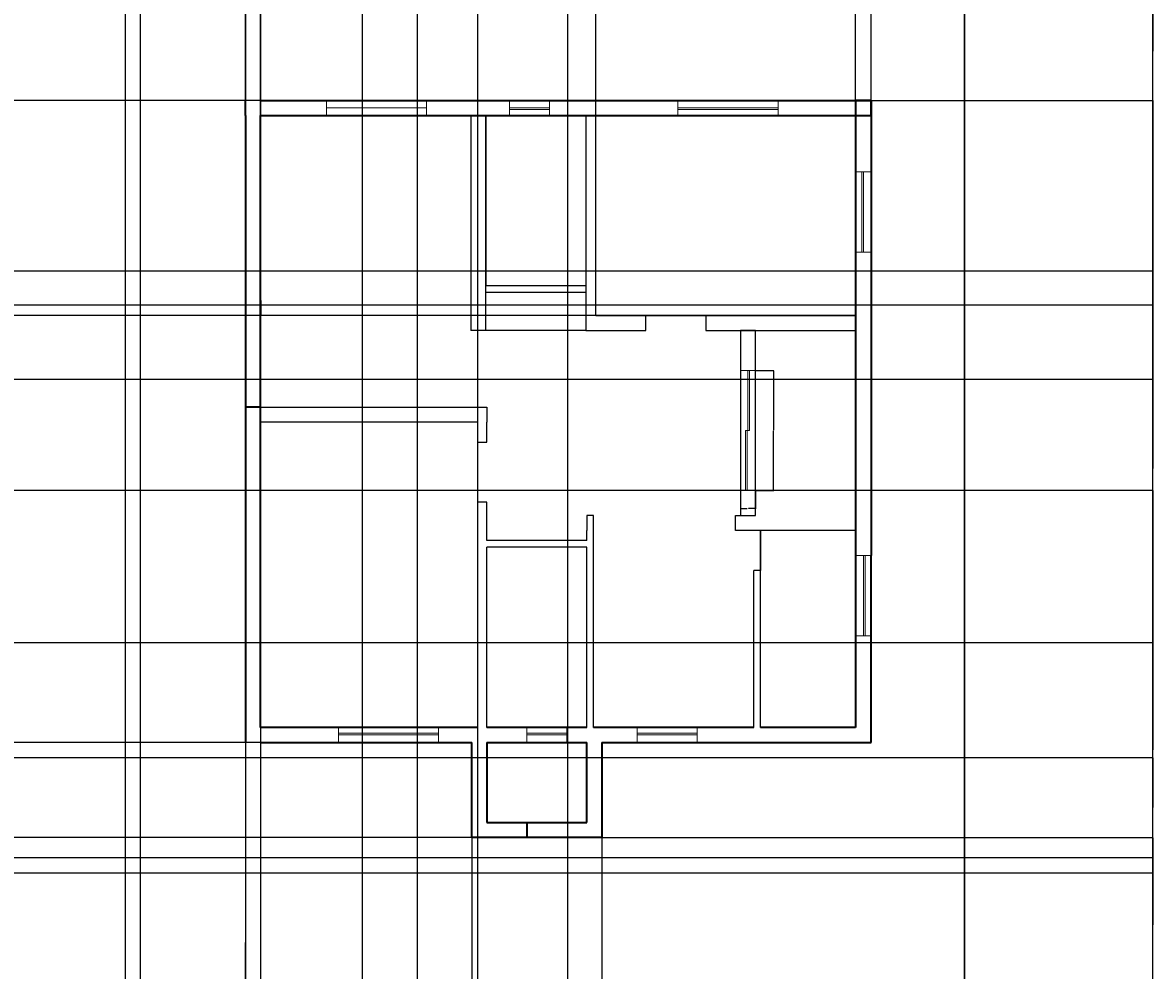
# Model space of a CAD drawing. Units: inches. Extents: x 2029 to 8798, y 1998 to 6373.
# Tile 7 of 11: x 3826 to 4504, y 4599 to 5168. Entities that reach past the tile are written whole.
import ezdxf

# ---------------------------------------------------------------- set-up
doc = ezdxf.new("R2010")
doc.units = ezdxf.units.IN
for name, color, linetype, lineweight in [('A-ANNO-DIMS', 2, 'Continuous', 18), ('A-GLAZ', 4, 'Continuous', 18), ('A-WALL-CIRC', 7, 'Continuous', 25), ('A-WALL-EXTR', 7, 'Continuous', 35), ('A-WALL-INTR', 7, 'Continuous', 25)]:
    doc.layers.add(name, color=color, linetype=linetype, lineweight=lineweight)
doc.styles.get("Standard").update_dxf_attribs({"font": 'arial.ttf'})
doc.dimstyles.get("Standard").update_dxf_attribs({"dimtxt": 0.18, "dimasz": 0.18, "dimexe": 0.18, "dimexo": 0.0625, "dimgap": 0.09, "dimtad": 0, "dimtih": 1, "dimtoh": 1, "dimdec": 4, "dimzin": 0, "dimdsep": 46, "dimtxsty": 'Standard', "dimcen": 0.09, "dimadec": 0, "dimazin": 0, "dimtfac": 1, "dimtdec": 4, "dimtofl": 0, "dimtmove": 0, "dimatfit": 3, "dimfxl": 1, "dimtolj": 1, "dimtzin": 0, "dimarcsym": 0})

# ---------------------------------------------------------------- blocks, each defined once
blk = doc.blocks.new('WIN-60')
for p, q in [((0, 0), (0, 9)), ((60, 9), (60, 0)), ((0, 4.5), (60, 4.5)), ((0, 3.5), (60, 3.5))]:
    blk.add_line(p, q)
blk = doc.blocks.new('WIN-36')
for p, q in [((0, 36), (9, 36)), ((3.5, 36), (3.5, 0)), ((4.5, 36), (4.5, 0)), ((9, 0), (0, 0))]:
    blk.add_line(p, q)
blk = doc.blocks.new('WIN-24')
for p, q in [((0, 0), (0, 9)), ((24, 9), (24, 0)), ((0, 4.5), (24, 4.5)), ((0, 3.5), (24, 3.5))]:
    blk.add_line(p, q)
blk = doc.blocks.new('WIN-48-DEEP-JAMB')
for p, q in [((9.38, 48), (0, 48)), ((0, 48), (0, 0)), ((3.69, 48), (3.69, 0)), ((4.69, 48), (4.69, 0)), ((0, 0), (9.38, 0))]:
    blk.add_line(p, q)
blk = doc.blocks.new('GLAZ-SLIDER-72-V')
for p, q in [((0, 72), (9, 72)), ((4.5, 72), (4.5, 36)), ((5.5, 72), (5.5, 36)), ((9, 72), (9, 0)), ((3, 36), (3, 0)), ((3, 36), (4, 36)), ((4, 36), (4, 0)), ((4.5, 36), (5.5, 36)), ((9, 0), (0, 0))]:
    blk.add_line(p, q)
blk = doc.blocks.new('WIN-60-SINGLE-LINE')
for p, q in [((0, 0), (0, 9)), ((0, 9), (60, 9)), ((60, 9), (60, 0)), ((0, 4.5), (60, 4.5))]:
    blk.add_line(p, q)
blk = doc.blocks.new('*D25')
at = {"layer": 'A-ANNO-DIMS', "color": 0, "lineweight": -2, "transparency": 16777216}
for p, q in [((4265.45, 4959.09), (4276.37, 4959.09)), ((4276.19, 4958.91), (4276.19, 4923.28)), ((4276.19, 4887.27), (4276.19, 4922.91)), ((4265.45, 4887.09), (4276.37, 4887.09))]:
    blk.add_line(p, q, dxfattribs=at)
at = {"layer": 'A-ANNO-DIMS', "color": 0, "transparency": 16777216}
for points in [[(4276.16, 4958.91), (4276.22, 4958.91), (4276.19, 4959.09)], [(4276.16, 4887.27), (4276.22, 4887.27), (4276.19, 4887.09)]]:
    blk.add_solid(points, dxfattribs=at)
at = {"layer": 'Defpoints', "color": 0, "transparency": 16777216}
for p in [(4265.39, 4959.09), (4276.19, 4959.09), (4265.39, 4887.09)]:
    blk.add_point(p, dxfattribs=at)
at = {"layer": 'A-ANNO-DIMS', "color": 0, "transparency": 16777216, "insert": (4276.19, 4923.09), "char_height": 0.18, "attachment_point": 5}
blk.add_mtext('\\A1;SLIDER 72 TYP.', dxfattribs=at)
blk = doc.blocks.new('*D26')
at = {"layer": 'A-ANNO-DIMS', "color": 0, "lineweight": -2, "transparency": 16777216}
for p, q in [((4256.39, 4887.03), (4256.39, 4876.11)), ((4265.39, 4887.03), (4265.39, 4876.11)), ((4256.57, 4876.29), (4260.43, 4876.29)), ((4265.21, 4876.29), (4261.35, 4876.29))]:
    blk.add_line(p, q, dxfattribs=at)
at = {"layer": 'A-ANNO-DIMS', "color": 0, "transparency": 16777216}
for points in [[(4256.57, 4876.32), (4256.57, 4876.26), (4256.39, 4876.29)], [(4265.21, 4876.32), (4265.21, 4876.26), (4265.39, 4876.29)]]:
    blk.add_solid(points, dxfattribs=at)
at = {"layer": 'Defpoints', "color": 0, "transparency": 16777216}
for p in [(4256.39, 4887.09), (4265.39, 4887.09), (4265.39, 4876.29)]:
    blk.add_point(p, dxfattribs=at)
at = {"layer": 'A-ANNO-DIMS', "color": 0, "transparency": 16777216, "insert": (4260.89, 4876.29), "char_height": 0.18, "attachment_point": 5}
blk.add_mtext('\\A1;9 TYP.', dxfattribs=at)
blk = doc.blocks.new('*D60')
at = {"layer": 'A-ANNO-DIMS', "color": 0, "lineweight": -2, "transparency": 16777216}
for p, q in [((3414.59, 5346.99), (4503.7, 5346.99)), ((4503.52, 5346.81), (4503.52, 5150.67)), ((4503.52, 4954.17), (4503.52, 5150.31)), ((3414.59, 4953.99), (4503.7, 4953.99))]:
    blk.add_line(p, q, dxfattribs=at)
at = {"layer": 'A-ANNO-DIMS', "color": 0, "transparency": 16777216}
for points in [[(4503.49, 5346.81), (4503.55, 5346.81), (4503.52, 5346.99)], [(4503.49, 4954.17), (4503.55, 4954.17), (4503.52, 4953.99)]]:
    blk.add_solid(points, dxfattribs=at)
at = {"layer": 'Defpoints', "color": 0, "transparency": 16777216}
for p in [(3414.53, 5346.99), (4503.52, 5346.99), (3414.53, 4953.99)]:
    blk.add_point(p, dxfattribs=at)
at = {"layer": 'A-ANNO-DIMS', "color": 0, "transparency": 16777216, "insert": (4503.52, 5150.49), "char_height": 0.18, "attachment_point": 5}
blk.add_mtext('\\A1;393', dxfattribs=at)
blk = doc.blocks.new('*D68')
at = {"layer": 'A-ANNO-DIMS', "color": 0, "lineweight": -2, "transparency": 16777216}
for p, q in [((3479.59, 4887.3), (4503.7, 4887.3)), ((4503.52, 4887.12), (4503.52, 4772.83)), ((4503.52, 4658.17), (4503.52, 4772.46)), ((3479.59, 4657.99), (4503.7, 4657.99))]:
    blk.add_line(p, q, dxfattribs=at)
at = {"layer": 'A-ANNO-DIMS', "color": 0, "transparency": 16777216}
for points in [[(4503.49, 4887.12), (4503.55, 4887.12), (4503.52, 4887.3)], [(4503.49, 4658.17), (4503.55, 4658.17), (4503.52, 4657.99)]]:
    blk.add_solid(points, dxfattribs=at)
at = {"layer": 'Defpoints', "color": 0, "transparency": 16777216}
for p in [(3479.53, 4887.3), (4503.52, 4887.3), (3479.53, 4657.99)]:
    blk.add_point(p, dxfattribs=at)
at = {"layer": 'A-ANNO-DIMS', "color": 0, "transparency": 16777216, "insert": (4503.52, 4772.64), "char_height": 0.18, "attachment_point": 5}
blk.add_mtext('\\A1;229.3', dxfattribs=at)
blk = doc.blocks.new('*D69')
at = {"layer": 'A-ANNO-DIMS', "color": 0, "lineweight": -2, "transparency": 16777216}
for p, q in [((3414.59, 4953.99), (4503.7, 4953.99)), ((4503.52, 4953.81), (4503.52, 4920.83)), ((4503.52, 4887.48), (4503.52, 4920.46)), ((3479.59, 4887.3), (4503.7, 4887.3))]:
    blk.add_line(p, q, dxfattribs=at)
at = {"layer": 'A-ANNO-DIMS', "color": 0, "transparency": 16777216}
for points in [[(4503.49, 4953.81), (4503.55, 4953.81), (4503.52, 4953.99)], [(4503.49, 4887.48), (4503.55, 4887.48), (4503.52, 4887.3)]]:
    blk.add_solid(points, dxfattribs=at)
at = {"layer": 'Defpoints', "color": 0, "transparency": 16777216}
for p in [(3414.53, 4953.99), (3479.53, 4887.3), (4503.52, 4887.3)]:
    blk.add_point(p, dxfattribs=at)
at = {"layer": 'A-ANNO-DIMS', "color": 0, "transparency": 16777216, "insert": (4503.52, 4920.64), "char_height": 0.18, "attachment_point": 5}
blk.add_mtext('\\A1;66.69', dxfattribs=at)
blk = doc.blocks.new('*D71')
at = {"layer": 'A-ANNO-DIMS', "color": 0, "lineweight": -2, "transparency": 16777216}
for p, q in [((4173.45, 4679.09), (4503.7, 4679.09)), ((4503.52, 4678.91), (4503.52, 4626.72)), ((4503.52, 4574.17), (4503.52, 4626.36)), ((4390.83, 4573.99), (4503.7, 4573.99))]:
    blk.add_line(p, q, dxfattribs=at)
at = {"layer": 'A-ANNO-DIMS', "color": 0, "transparency": 16777216}
for points in [[(4503.49, 4678.91), (4503.55, 4678.91), (4503.52, 4679.09)], [(4503.49, 4574.17), (4503.55, 4574.17), (4503.52, 4573.99)]]:
    blk.add_solid(points, dxfattribs=at)
at = {"layer": 'Defpoints', "color": 0, "transparency": 16777216}
for p in [(4173.39, 4679.09), (4503.52, 4679.09), (4390.77, 4573.99)]:
    blk.add_point(p, dxfattribs=at)
at = {"layer": 'A-ANNO-DIMS', "color": 0, "transparency": 16777216, "insert": (4503.52, 4626.54), "char_height": 0.18, "attachment_point": 5}
blk.add_mtext('\\A1;105.1', dxfattribs=at)
blk = doc.blocks.new('*D72')
at = {"layer": 'A-ANNO-DIMS', "color": 0, "lineweight": -2, "transparency": 16777216}
for p, q in [((4334.83, 5121.09), (4503.7, 5121.09)), ((4503.52, 5120.91), (4503.52, 4900.28)), ((4503.52, 4679.27), (4503.52, 4899.91)), ((4173.45, 4679.09), (4503.7, 4679.09))]:
    blk.add_line(p, q, dxfattribs=at)
at = {"layer": 'A-ANNO-DIMS', "color": 0, "transparency": 16777216}
for points in [[(4503.49, 5120.91), (4503.55, 5120.91), (4503.52, 5121.09)], [(4503.49, 4679.27), (4503.55, 4679.27), (4503.52, 4679.09)]]:
    blk.add_solid(points, dxfattribs=at)
at = {"layer": 'Defpoints', "color": 0, "transparency": 16777216}
for p in [(4334.77, 5121.09), (4503.52, 5121.09), (4173.39, 4679.09)]:
    blk.add_point(p, dxfattribs=at)
at = {"layer": 'A-ANNO-DIMS', "color": 0, "transparency": 16777216, "insert": (4503.52, 4900.09), "char_height": 0.18, "attachment_point": 5}
blk.add_mtext('\\A1;442', dxfattribs=at)
blk = doc.blocks.new('*D73')
at = {"layer": 'A-ANNO-DIMS', "color": 0, "lineweight": -2, "transparency": 16777216}
for p, q in [((4173.45, 5230.61), (4503.7, 5230.61)), ((4503.52, 5230.43), (4503.52, 5176.04)), ((4503.52, 5121.27), (4503.52, 5175.67)), ((4334.83, 5121.09), (4503.7, 5121.09))]:
    blk.add_line(p, q, dxfattribs=at)
at = {"layer": 'A-ANNO-DIMS', "color": 0, "transparency": 16777216}
for points in [[(4503.49, 5230.43), (4503.55, 5230.43), (4503.52, 5230.61)], [(4503.49, 5121.27), (4503.55, 5121.27), (4503.52, 5121.09)]]:
    blk.add_solid(points, dxfattribs=at)
at = {"layer": 'Defpoints', "color": 0, "transparency": 16777216}
for p in [(4173.39, 5230.61), (4503.52, 5230.61), (4334.77, 5121.09)]:
    blk.add_point(p, dxfattribs=at)
at = {"layer": 'A-ANNO-DIMS', "color": 0, "transparency": 16777216, "insert": (4503.52, 5175.85), "char_height": 0.18, "attachment_point": 5}
blk.add_mtext('\\A1;109.52', dxfattribs=at)
blk = doc.blocks.new('*D76')
at = {"layer": 'A-ANNO-DIMS', "color": 0, "lineweight": -2, "transparency": 16777216}
for p, q in [((3887.77, 5813.55), (3887.77, 4031.06)), ((4390.77, 5813.55), (4390.77, 4031.06)), ((3887.95, 4031.24), (4138.98, 4031.24)), ((4390.59, 4031.24), (4139.55, 4031.24))]:
    blk.add_line(p, q, dxfattribs=at)
at = {"layer": 'A-ANNO-DIMS', "color": 0, "transparency": 16777216}
for points in [[(3887.95, 4031.27), (3887.95, 4031.21), (3887.77, 4031.24)], [(4390.59, 4031.27), (4390.59, 4031.21), (4390.77, 4031.24)]]:
    blk.add_solid(points, dxfattribs=at)
at = {"layer": 'Defpoints', "color": 0, "transparency": 16777216}
for p in [(3887.77, 5813.61), (4390.77, 5813.61), (4390.77, 4031.24)]:
    blk.add_point(p, dxfattribs=at)
at = {"layer": 'A-ANNO-DIMS', "color": 0, "transparency": 16777216, "insert": (4139.27, 4031.24), "char_height": 0.18, "attachment_point": 5}
blk.add_mtext('\\A1;503', dxfattribs=at)
blk = doc.blocks.new('*D77')
at = {"layer": 'A-ANNO-DIMS', "color": 0, "lineweight": -2, "transparency": 16777216}
for p, q in [((3959.77, 5121.16), (3959.77, 6372.54)), ((3959.95, 6372.36), (4146.98, 6372.36)), ((4334.59, 6372.36), (4147.56, 6372.36)), ((4334.77, 5121.16), (4334.77, 6372.54))]:
    blk.add_line(p, q, dxfattribs=at)
at = {"layer": 'A-ANNO-DIMS', "color": 0, "transparency": 16777216}
for points in [[(3959.95, 6372.39), (3959.95, 6372.33), (3959.77, 6372.36)], [(4334.59, 6372.39), (4334.59, 6372.33), (4334.77, 6372.36)]]:
    blk.add_solid(points, dxfattribs=at)
at = {"layer": 'Defpoints', "color": 0, "transparency": 16777216}
for p in [(4334.77, 6372.36), (3959.77, 5121.09), (4334.77, 5121.09)]:
    blk.add_point(p, dxfattribs=at)
at = {"layer": 'A-ANNO-DIMS', "color": 0, "transparency": 16777216, "insert": (4147.27, 6372.36), "char_height": 0.18, "attachment_point": 5}
blk.add_mtext('\\A1;375', dxfattribs=at)
blk = doc.blocks.new('*D78')
at = {"layer": 'A-ANNO-DIMS', "color": 0, "lineweight": -2, "transparency": 16777216}
for p, q in [((3896.77, 6211.55), (3896.77, 4031.06)), ((4029.77, 6211.55), (4029.77, 4031.06)), ((3896.95, 4031.24), (3962.99, 4031.24)), ((4029.59, 4031.24), (3963.55, 4031.24))]:
    blk.add_line(p, q, dxfattribs=at)
at = {"layer": 'A-ANNO-DIMS', "color": 0, "transparency": 16777216}
for points in [[(3896.95, 4031.27), (3896.95, 4031.21), (3896.77, 4031.24)], [(4029.59, 4031.27), (4029.59, 4031.21), (4029.77, 4031.24)]]:
    blk.add_solid(points, dxfattribs=at)
at = {"layer": 'Defpoints', "color": 0, "transparency": 16777216}
for p in [(3896.77, 6211.61), (4029.77, 6211.61), (4029.77, 4031.24)]:
    blk.add_point(p, dxfattribs=at)
at = {"layer": 'A-ANNO-DIMS', "color": 0, "transparency": 16777216, "insert": (3963.27, 4031.24), "char_height": 0.18, "attachment_point": 5}
blk.add_mtext('\\A1;133', dxfattribs=at)
blk = doc.blocks.new('*D83')
at = {"layer": 'A-ANNO-DIMS', "color": 0, "lineweight": -2, "transparency": 16777216}
for p, q in [((4062.77, 6151.55), (4062.77, 4031.06)), ((4152.77, 6151.55), (4152.77, 4031.06)), ((4062.95, 4031.24), (4107.55, 4031.24)), ((4152.59, 4031.24), (4107.98, 4031.24))]:
    blk.add_line(p, q, dxfattribs=at)
at = {"layer": 'A-ANNO-DIMS', "color": 0, "transparency": 16777216}
for points in [[(4062.95, 4031.27), (4062.95, 4031.21), (4062.77, 4031.24)], [(4152.59, 4031.27), (4152.59, 4031.21), (4152.77, 4031.24)]]:
    blk.add_solid(points, dxfattribs=at)
at = {"layer": 'Defpoints', "color": 0, "transparency": 16777216}
for p in [(4062.77, 6151.61), (4152.77, 6151.61), (4152.77, 4031.24)]:
    blk.add_point(p, dxfattribs=at)
at = {"layer": 'A-ANNO-DIMS', "color": 0, "transparency": 16777216, "insert": (4107.77, 4031.24), "char_height": 0.18, "attachment_point": 5}
blk.add_mtext('\\A1;90', dxfattribs=at)
blk = doc.blocks.new('*D88')
at = {"layer": 'A-ANNO-DIMS', "color": 0, "lineweight": -2, "transparency": 16777216}
for p, q in [((2142.54, 4445.05), (2142.54, 6372.54)), ((2142.72, 6372.36), (3266.19, 6372.36)), ((4390.59, 6372.36), (3267.12, 6372.36)), ((4390.77, 4574.05), (4390.77, 6372.54))]:
    blk.add_line(p, q, dxfattribs=at)
at = {"layer": 'A-ANNO-DIMS', "color": 0, "transparency": 16777216}
for points in [[(2142.72, 6372.39), (2142.72, 6372.33), (2142.54, 6372.36)], [(4390.59, 6372.39), (4390.59, 6372.33), (4390.77, 6372.36)]]:
    blk.add_solid(points, dxfattribs=at)
at = {"layer": 'Defpoints', "color": 0, "transparency": 16777216}
for p in [(4390.77, 6372.36), (4390.77, 4573.99), (2142.54, 4444.99)]:
    blk.add_point(p, dxfattribs=at)
at = {"layer": 'A-ANNO-DIMS', "color": 0, "transparency": 16777216, "insert": (3266.65, 6372.36), "char_height": 0.18, "attachment_point": 5}
blk.add_mtext('\\A1;2248.2', dxfattribs=at)
blk = doc.blocks.new('*D89')
at = {"layer": 'A-ANNO-DIMS', "color": 0, "lineweight": -2, "transparency": 16777216}
for p, q in [((4249.83, 6259.61), (4503.7, 6259.61)), ((4503.52, 6259.43), (4503.52, 5201.98)), ((4503.52, 4144.17), (4503.52, 5201.62)), ((4105.83, 4143.99), (4503.7, 4143.99))]:
    blk.add_line(p, q, dxfattribs=at)
at = {"layer": 'A-ANNO-DIMS', "color": 0, "transparency": 16777216}
for points in [[(4503.49, 6259.43), (4503.55, 6259.43), (4503.52, 6259.61)], [(4503.49, 4144.17), (4503.55, 4144.17), (4503.52, 4143.99)]]:
    blk.add_solid(points, dxfattribs=at)
at = {"layer": 'Defpoints', "color": 0, "transparency": 16777216}
for p in [(4249.77, 6259.61), (4503.52, 6259.61), (4105.77, 4143.99)]:
    blk.add_point(p, dxfattribs=at)
at = {"layer": 'A-ANNO-DIMS', "color": 0, "transparency": 16777216, "insert": (4503.52, 5201.8), "char_height": 0.18, "attachment_point": 5}
blk.add_mtext('\\A1;2115.6', dxfattribs=at)
blk = doc.blocks.new('*D90')
at = {"layer": 'A-ANNO-DIMS', "color": 0, "lineweight": -2, "transparency": 16777216}
for p, q in [((4095.39, 4679.03), (4095.39, 4031.06)), ((4173.39, 4679.03), (4173.39, 4031.06)), ((4095.57, 4031.24), (4134.17, 4031.24)), ((4173.21, 4031.24), (4134.61, 4031.24))]:
    blk.add_line(p, q, dxfattribs=at)
at = {"layer": 'A-ANNO-DIMS', "color": 0, "transparency": 16777216}
for points in [[(4095.57, 4031.27), (4095.57, 4031.21), (4095.39, 4031.24)], [(4173.21, 4031.27), (4173.21, 4031.21), (4173.39, 4031.24)]]:
    blk.add_solid(points, dxfattribs=at)
at = {"layer": 'Defpoints', "color": 0, "transparency": 16777216}
for p in [(4095.39, 4679.09), (4173.39, 4679.09), (4173.39, 4031.24)]:
    blk.add_point(p, dxfattribs=at)
at = {"layer": 'A-ANNO-DIMS', "color": 0, "transparency": 16777216, "insert": (4134.39, 4031.24), "char_height": 0.18, "attachment_point": 5}
blk.add_mtext('\\A1;78', dxfattribs=at)
blk = doc.blocks.new('*D91')
at = {"layer": 'A-ANNO-DIMS', "color": 0, "lineweight": -2, "transparency": 16777216}
for p, q in [((4095.32, 4736.09), (2029.61, 4736.09)), ((2029.79, 4735.91), (2029.79, 4707.78)), ((2029.79, 4679.27), (2029.79, 4707.41)), ((4095.32, 4679.09), (2029.61, 4679.09))]:
    blk.add_line(p, q, dxfattribs=at)
at = {"layer": 'A-ANNO-DIMS', "color": 0, "transparency": 16777216}
for points in [[(2029.76, 4735.91), (2029.82, 4735.91), (2029.79, 4736.09)], [(2029.76, 4679.27), (2029.82, 4679.27), (2029.79, 4679.09)]]:
    blk.add_solid(points, dxfattribs=at)
at = {"layer": 'Defpoints', "color": 0, "transparency": 16777216}
for p in [(2029.79, 4736.09), (4095.39, 4736.09), (4095.39, 4679.09)]:
    blk.add_point(p, dxfattribs=at)
at = {"layer": 'A-ANNO-DIMS', "color": 0, "transparency": 16777216, "insert": (2029.79, 4707.59), "char_height": 0.18, "attachment_point": 5}
blk.add_mtext('\\A1;57', dxfattribs=at)
blk = doc.blocks.new('*D92')
at = {"layer": 'A-ANNO-DIMS', "color": 0, "lineweight": -2, "transparency": 16777216}
for p, q in [((3959.77, 4736.03), (3959.77, 4031.06)), ((4095.39, 4679.03), (4095.39, 4031.06)), ((3959.95, 4031.24), (4027.12, 4031.24)), ((4095.21, 4031.24), (4028.03, 4031.24))]:
    blk.add_line(p, q, dxfattribs=at)
at = {"layer": 'A-ANNO-DIMS', "color": 0, "transparency": 16777216}
for points in [[(3959.95, 4031.27), (3959.95, 4031.21), (3959.77, 4031.24)], [(4095.21, 4031.27), (4095.21, 4031.21), (4095.39, 4031.24)]]:
    blk.add_solid(points, dxfattribs=at)
at = {"layer": 'Defpoints', "color": 0, "transparency": 16777216}
for p in [(3959.77, 4736.09), (4095.39, 4679.09), (4095.39, 4031.24)]:
    blk.add_point(p, dxfattribs=at)
at = {"layer": 'A-ANNO-DIMS', "color": 0, "transparency": 16777216, "insert": (4027.58, 4031.24), "char_height": 0.18, "attachment_point": 5}
blk.add_mtext('\\A1;135.62', dxfattribs=at)
blk = doc.blocks.new('*D106')
at = {"layer": 'A-ANNO-DIMS', "color": 0, "lineweight": -2, "transparency": 16777216}
for p, q in [((4325.32, 5121.09), (2029.61, 5121.09)), ((2029.79, 5120.91), (2029.79, 5056.78)), ((2029.79, 4992.27), (2029.79, 5056.41)), ((4325.32, 4992.09), (2029.61, 4992.09))]:
    blk.add_line(p, q, dxfattribs=at)
at = {"layer": 'A-ANNO-DIMS', "color": 0, "transparency": 16777216}
for points in [[(2029.76, 5120.91), (2029.82, 5120.91), (2029.79, 5121.09)], [(2029.76, 4992.27), (2029.82, 4992.27), (2029.79, 4992.09)]]:
    blk.add_solid(points, dxfattribs=at)
at = {"layer": 'Defpoints', "color": 0, "transparency": 16777216}
for p in [(4325.39, 5121.09), (2029.79, 4992.09), (4325.39, 4992.09)]:
    blk.add_point(p, dxfattribs=at)
at = {"layer": 'A-ANNO-DIMS', "color": 0, "transparency": 16777216, "insert": (2029.79, 5056.59), "char_height": 0.18, "attachment_point": 5}
blk.add_mtext('\\A1;129', dxfattribs=at)
blk = doc.blocks.new('*D107')
at = {"layer": 'A-ANNO-DIMS', "color": 0, "lineweight": -2, "transparency": 16777216}
for p, q in [((3968.77, 5479.55), (3968.77, 4031.06)), ((4098.77, 5479.55), (4098.77, 4031.06)), ((3968.95, 4031.24), (4033.49, 4031.24)), ((4098.59, 4031.24), (4034.05, 4031.24))]:
    blk.add_line(p, q, dxfattribs=at)
at = {"layer": 'A-ANNO-DIMS', "color": 0, "transparency": 16777216}
for points in [[(3968.95, 4031.27), (3968.95, 4031.21), (3968.77, 4031.24)], [(4098.59, 4031.27), (4098.59, 4031.21), (4098.77, 4031.24)]]:
    blk.add_solid(points, dxfattribs=at)
at = {"layer": 'Defpoints', "color": 0, "transparency": 16777216}
for p in [(3968.77, 5479.61), (4098.77, 5479.61), (4098.77, 4031.24)]:
    blk.add_point(p, dxfattribs=at)
at = {"layer": 'A-ANNO-DIMS', "color": 0, "transparency": 16777216, "insert": (4033.77, 4031.24), "char_height": 0.18, "attachment_point": 5}
blk.add_mtext('\\A1;130', dxfattribs=at)
blk = doc.blocks.new('*D109')
at = {"layer": 'A-ANNO-DIMS', "color": 0, "lineweight": -2, "transparency": 16777216}
for p, q in [((4169.77, 4992.16), (4169.77, 6372.54)), ((4169.95, 6372.36), (4247.12, 6372.36)), ((4325.21, 6372.36), (4248.03, 6372.36)), ((4325.39, 4992.16), (4325.39, 6372.54))]:
    blk.add_line(p, q, dxfattribs=at)
at = {"layer": 'A-ANNO-DIMS', "color": 0, "transparency": 16777216}
for points in [[(4169.95, 6372.39), (4169.95, 6372.33), (4169.77, 6372.36)], [(4325.21, 6372.39), (4325.21, 6372.33), (4325.39, 6372.36)]]:
    blk.add_solid(points, dxfattribs=at)
at = {"layer": 'Defpoints', "color": 0, "transparency": 16777216}
for p in [(4325.39, 6372.36), (4169.77, 4992.09), (4325.39, 4992.09)]:
    blk.add_point(p, dxfattribs=at)
at = {"layer": 'A-ANNO-DIMS', "color": 0, "transparency": 16777216, "insert": (4247.58, 6372.36), "char_height": 0.18, "attachment_point": 5}
blk.add_mtext('\\A1;155.62', dxfattribs=at)
blk = doc.blocks.new('*D110')
at = {"layer": 'A-ANNO-DIMS', "color": 0, "lineweight": -2, "transparency": 16777216}
for p, q in [((2723.6, 5018.96), (4503.7, 5018.96)), ((4503.52, 5018.78), (4503.52, 5008.93)), ((4503.52, 4998.71), (4503.52, 5008.56)), ((2723.6, 4998.53), (4503.7, 4998.53))]:
    blk.add_line(p, q, dxfattribs=at)
at = {"layer": 'A-ANNO-DIMS', "color": 0, "transparency": 16777216}
for points in [[(4503.49, 5018.78), (4503.55, 5018.78), (4503.52, 5018.96)], [(4503.49, 4998.71), (4503.55, 4998.71), (4503.52, 4998.53)]]:
    blk.add_solid(points, dxfattribs=at)
at = {"layer": 'Defpoints', "color": 0, "transparency": 16777216}
for p in [(2723.54, 5018.96), (2723.54, 4998.53), (4503.52, 4998.53)]:
    blk.add_point(p, dxfattribs=at)
at = {"layer": 'A-ANNO-DIMS', "color": 0, "transparency": 16777216, "insert": (4503.52, 5008.75), "char_height": 0.18, "attachment_point": 5}
blk.add_mtext('\\A1;20.425', dxfattribs=at)
blk = doc.blocks.new('*D111')
at = {"layer": 'A-ANNO-DIMS', "color": 0, "lineweight": -2, "transparency": 16777216}
for p, q in [((2723.6, 4726.96), (4503.7, 4726.96)), ((4503.52, 4726.78), (4503.52, 4697.16)), ((4503.52, 4667.17), (4503.52, 4696.79)), ((2723.6, 4666.99), (4503.7, 4666.99))]:
    blk.add_line(p, q, dxfattribs=at)
at = {"layer": 'A-ANNO-DIMS', "color": 0, "transparency": 16777216}
for points in [[(4503.49, 4726.78), (4503.55, 4726.78), (4503.52, 4726.96)], [(4503.49, 4667.17), (4503.55, 4667.17), (4503.52, 4666.99)]]:
    blk.add_solid(points, dxfattribs=at)
at = {"layer": 'Defpoints', "color": 0, "transparency": 16777216}
for p in [(2723.54, 4726.96), (4503.52, 4726.96), (2723.54, 4666.99)]:
    blk.add_point(p, dxfattribs=at)
at = {"layer": 'A-ANNO-DIMS', "color": 0, "transparency": 16777216, "insert": (4503.52, 4696.97), "char_height": 0.18, "attachment_point": 5}
blk.add_mtext('\\A1;59.97', dxfattribs=at)
blk = doc.blocks.new('*D113')
at = {"layer": 'A-ANNO-DIMS', "color": 0, "lineweight": -2, "transparency": 16777216}
for p, q in [((2864.59, 4795.99), (4503.7, 4795.99)), ((4503.52, 4795.81), (4503.52, 4731.67)), ((4503.52, 4667.17), (4503.52, 4731.31)), ((2864.59, 4666.99), (4503.7, 4666.99))]:
    blk.add_line(p, q, dxfattribs=at)
at = {"layer": 'A-ANNO-DIMS', "color": 0, "transparency": 16777216}
for points in [[(4503.49, 4795.81), (4503.55, 4795.81), (4503.52, 4795.99)], [(4503.49, 4667.17), (4503.55, 4667.17), (4503.52, 4666.99)]]:
    blk.add_solid(points, dxfattribs=at)
at = {"layer": 'Defpoints', "color": 0, "transparency": 16777216}
for p in [(2864.53, 4795.99), (4503.52, 4795.99), (2864.53, 4666.99)]:
    blk.add_point(p, dxfattribs=at)
at = {"layer": 'A-ANNO-DIMS', "color": 0, "transparency": 16777216, "insert": (4503.52, 4731.49), "char_height": 0.18, "attachment_point": 5}
blk.add_mtext('\\A1;129', dxfattribs=at)

msp = doc.modelspace()

# ---------------------------------------------------------------- linework, layer by layer
at = {"layer": 'A-GLAZ'}
for p, q in [((4118.0329, 5121.0948), (4142.0329, 5121.0948)), ((4218.9796, 5121.0948), (4278.9796, 5121.0948)), ((4075.4621, 4736.0948), (4015.4621, 4736.0948)), ((4152.3869, 4736.0948), (4128.3869, 4736.0948)), ((4230.5315, 4736.0948), (4194.5315, 4736.0948))]:
    msp.add_line(p, q, dxfattribs=at)
at = {"layer": 'A-WALL-CIRC'}
for p, q in [((3959.7657, 5287.6123), (3959.7657, 5167.6123)), ((3968.7657, 5107.6123), (3968.7657, 5287.6123)), ((3959.7657, 5167.6123), (3959.7657, 5107.6123)), ((3959.7657, 4736.0948), (3959.7657, 4616.0948)), ((3968.7657, 4736.0948), (3968.7657, 4573.9886)), ((3959.7657, 4573.9886), (3959.7657, 4616.0948))]:
    msp.add_line(p, q, dxfattribs=at)
at = {"layer": 'A-WALL-EXTR'}
for p, q in [((3959.7657, 5112.0948), (3959.7657, 5121.0948)), ((3968.7657, 5121.0948), (4334.3869, 5121.0948)), ((4334.3869, 5121.0948), (4325.3869, 5121.0948)), ((4325.3869, 5121.0948), (4325.3869, 4848.0948)), ((4334.7657, 5121.0948), (4332.4986, 5121.0948)), ((4334.7657, 5112.0948), (4334.7657, 5121.0948)), ((4334.7657, 5121.0948), (4334.7657, 4848.0948)), ((3959.7657, 5112.0948), (3959.7657, 4736.0948)), ((3968.7657, 4992.0948), (3968.7657, 5112.0948)), ((3968.7657, 5112.0948), (4094.7657, 5112.0948)), ((3968.7657, 5112.0948), (4008.3833, 5112.0948)), ((3968.7657, 5112.0948), (4094.7657, 5112.0948)), ((3991.2657, 5112.0948), (4097.1962, 5112.0948)), ((4094.7657, 5112.0948), (4334.7657, 5112.0948)), ((4103.7657, 5112.0948), (4163.7657, 5112.0948)), ((4103.7657, 5112.0948), (4118.0329, 5112.0948)), ((4169.7657, 5112.0948), (4218.9796, 5112.0948)), ((4334.7657, 5112.0948), (4334.7657, 5078.1445)), ((3968.7657, 5001.0948), (3968.7657, 4992.0948)), ((3968.7657, 4745.0948), (3968.7657, 4992.0948)), ((4325.3869, 4983.0948), (4325.3869, 4863.0948)), ((3968.7657, 4937.0948), (3959.7657, 4937.0948)), ((3968.7657, 4937.0948), (3968.7657, 4937.0948)), ((3968.7657, 4928.0948), (3968.7657, 4937.0948)), ((3968.7657, 4745.0948), (3968.7657, 4928.0948)), ((4325.3869, 4863.0948), (4325.3869, 4745.0948)), ((4334.7657, 4745.0948), (4334.7657, 4848.0948)), ((3968.7657, 4745.0948), (3968.7657, 4745.0948)), ((4098.7657, 4745.0948), (3968.7657, 4745.0948)), ((4098.7657, 4745.0948), (4075.4621, 4745.0948)), ((4164.3869, 4745.0948), (4104.3869, 4745.0948)), ((4160.3869, 4745.0948), (4104.3869, 4745.0948)), ((4164.3869, 4745.0948), (4104.3869, 4745.0948)), ((4164.3869, 4745.0948), (4104.3869, 4745.0948)), ((4164.3869, 4745.0948), (4152.3869, 4745.0948)), ((4262.3869, 4745.0948), (4168.3869, 4745.0948)), ((4262.3869, 4745.0948), (4168.3869, 4745.0948)), ((4262.3869, 4745.0948), (4230.5315, 4745.0948)), ((4264.3869, 4745.0948), (4262.3869, 4745.0948)), ((4325.3869, 4745.0948), (4268.3869, 4745.0948)), ((4325.3869, 4745.0948), (4268.3869, 4745.0948)), ((4334.7657, 4736.0948), (4334.7657, 4745.0948)), ((3968.7657, 4736.0948), (4095.3869, 4736.0948)), ((4095.3869, 4679.0948), (4095.3869, 4736.0948)), ((4104.3869, 4736.0948), (4104.3869, 4688.0948)), ((4104.3869, 4736.0948), (4164.3869, 4736.0948)), ((4164.3869, 4688.0948), (4164.3869, 4736.0948)), ((4173.3869, 4736.0948), (4173.3869, 4679.0948)), ((4173.3869, 4736.0948), (4334.7657, 4736.0948)), ((4104.3869, 4688.0948), (4128.3869, 4688.0948)), ((4128.3869, 4688.0948), (4128.3869, 4679.0948)), ((4128.3869, 4688.0948), (4164.3869, 4688.0948)), ((4104.3869, 4679.0948), (4095.3869, 4679.0948)), ((4128.3869, 4679.0948), (4104.3869, 4679.0948)), ((4173.3869, 4679.0948), (4128.3869, 4679.0948))]:
    msp.add_line(p, q, dxfattribs=at)
at = {"layer": 'A-WALL-INTR'}
for p, q in [((4094.7657, 5112.0948), (4094.7657, 4983.0948)), ((4103.7657, 4983.0948), (4103.7657, 5112.0948)), ((4103.7657, 5112.0948), (4103.7657, 5010.0948)), ((4163.7657, 5112.0948), (4163.7657, 4992.0948)), ((4169.7657, 4992.0948), (4169.7657, 5112.0948)), ((4103.7657, 5010.0948), (4163.7657, 5010.0948)), ((4103.7657, 5006.0948), (4163.7657, 5006.0948)), ((4163.7657, 4992.0948), (4163.7657, 4983.0948)), ((4169.7657, 4992.0948), (4325.3869, 4992.0948)), ((4199.7657, 4983.0948), (4199.7657, 4992.0948)), ((4199.7657, 4992.0948), (4235.7657, 4992.0948)), ((4235.7657, 4992.0948), (4235.7657, 4983.0948)), ((4103.7657, 4983.0948), (4094.7657, 4983.0948)), ((4163.7657, 4983.0948), (4103.7657, 4983.0948)), ((4163.7657, 4983.0948), (4169.7657, 4983.0948)), ((4163.7657, 4983.0948), (4199.7657, 4983.0948)), ((4169.7657, 4983.0948), (4199.7657, 4983.0948)), ((4235.7657, 4983.0948), (4325.3869, 4983.0948)), ((4265.3869, 4983.0948), (4256.3869, 4983.0948)), ((4256.3869, 4983.0948), (4256.3869, 4872.0948)), ((4256.3869, 4983.0948), (4256.3869, 4959.0948)), ((4265.3869, 4872.0948), (4265.3869, 4983.0948)), ((3968.7657, 4937.0948), (4104.3869, 4937.0948)), ((4104.3869, 4937.0948), (4104.3869, 4928.0948)), ((4098.7657, 4928.0948), (3968.7657, 4928.0948)), ((4098.7657, 4928.0948), (4098.7657, 4745.0948)), ((4098.7657, 4928.0948), (4098.7657, 4916.0948)), ((4104.3869, 4916.0948), (4104.3869, 4928.0948)), ((4098.7657, 4916.0948), (4104.3869, 4916.0948)), ((4104.3869, 4880.0948), (4098.7657, 4880.0948)), ((4104.3869, 4857.0948), (4104.3869, 4880.0948)), ((4168.3869, 4872.0948), (4164.3869, 4872.0948)), ((4164.3869, 4872.0948), (4164.3869, 4863.0948)), ((4168.3869, 4863.0948), (4168.3869, 4872.0948)), ((4253.3869, 4863.0948), (4253.3869, 4872.0948)), ((4253.3869, 4872.0948), (4265.3869, 4872.0948)), ((4164.3869, 4857.0948), (4164.3869, 4863.0948)), ((4168.3869, 4745.0948), (4168.3869, 4863.0948)), ((4325.3869, 4863.0948), (4253.3869, 4863.0948)), ((4268.3869, 4863.0948), (4264.3869, 4863.0948)), ((4268.3869, 4745.0948), (4268.3869, 4863.0948)), ((4268.3869, 4863.0948), (4268.3869, 4839.0948)), ((4164.3869, 4857.0948), (4104.3869, 4857.0948)), ((4104.3869, 4745.0948), (4104.3869, 4853.0948)), ((4164.3869, 4853.0948), (4104.3869, 4853.0948)), ((4164.3869, 4745.0948), (4164.3869, 4853.0948)), ((4164.3869, 4745.0948), (4164.3869, 4853.0948)), ((4264.3869, 4745.0948), (4264.3869, 4839.0948)), ((4268.3869, 4839.0948), (4264.3869, 4839.0948))]:
    msp.add_line(p, q, dxfattribs=at)

# ---------------------------------------------------------------- block references
at = {"layer": 'A-GLAZ'}
for name, p in [('WIN-60-SINGLE-LINE', (4008.3833, 5112.0948)), ('WIN-24', (4118.0329, 5112.0948)), ('WIN-60', (4218.9796, 5112.0948)), ('WIN-48-DEEP-JAMB', (4325.3869, 5030.1445)), ('GLAZ-SLIDER-72-V', (4256.3869, 4887.0948))]:
    msp.add_blockref(name, p, dxfattribs=at)
at = {"layer": 'A-GLAZ', "extrusion": (0, 0, -1), "zscale": -1}
msp.add_blockref('WIN-48-DEEP-JAMB', (-4334.7657, 4800.0948), dxfattribs=at)
at = {"layer": 'A-GLAZ', "extrusion": (0, 0, -1), "zscale": -1, "rotation": 180}
for name, p in [('WIN-60', (-4015.4621, 4745.0948)), ('WIN-24', (-4128.3869, 4745.0948))]:
    msp.add_blockref(name, p, dxfattribs=at)
at = {"layer": 'A-GLAZ', "rotation": 270}
msp.add_blockref('WIN-36', (4194.5315, 4745.0948), dxfattribs=at)

# ---------------------------------------------------------------- dimensions: what is measured, and where the dimension line sits
at = {"layer": 'A-ANNO-DIMS'}
for base, p1, p2, override, picture, middle in [((4390.7657, 6372.3623), (2142.5398, 4444.9886), (4390.7657, 4573.9886), {"dimdec": 1, "dimlfac": 1, "dimrnd": 0, "dimzin": 0, "dimdsep": 46, "dimlunit": 2}, '*D88', (3266.6528, 6372.3623)), ((4334.7657, 6372.3623), (3959.7657, 5121.0948), (4334.7657, 5121.0948), {"dimdec": 0, "dimlfac": 1, "dimrnd": 0, "dimzin": 0, "dimdsep": 46, "dimlunit": 2}, '*D77', (4147.2657, 6372.3623)), ((4325.3869, 6372.3623), (4169.7657, 4992.0948), (4325.3869, 4992.0948), {"dimdec": 2, "dimlfac": 1, "dimrnd": 0, "dimzin": 0, "dimdsep": 46, "dimlunit": 2}, '*D109', (4247.5763, 6372.3623)), ((4029.7657, 4031.2386), (3896.7657, 6211.6123), (4029.7657, 6211.6123), {"dimdec": 0, "dimlfac": 1, "dimrnd": 0, "dimzin": 0, "dimdsep": 46, "dimlunit": 2}, '*D78', (3963.2657, 4031.2386)), ((4152.7657, 4031.2386), (4062.7657, 6151.6123), (4152.7657, 6151.6123), {"dimdec": 0, "dimlfac": 1, "dimrnd": 0, "dimzin": 0, "dimdsep": 46, "dimlunit": 2}, '*D83', (4107.7657, 4031.2386)), ((4390.7657, 4031.2386), (3887.7657, 5813.6123), (4390.7657, 5813.6123), {"dimdec": 0, "dimlfac": 1, "dimrnd": 0, "dimzin": 0, "dimdsep": 46, "dimlunit": 2}, '*D76', (4139.2657, 4031.2386)), ((4098.7657, 4031.2386), (3968.7657, 5479.6123), (4098.7657, 5479.6123), {"dimdec": 0, "dimlfac": 1, "dimrnd": 0, "dimzin": 0, "dimdsep": 46, "dimlunit": 2}, '*D107', (4033.7657, 4031.2386)), ((4095.3869, 4031.2386), (3959.7657, 4736.0948), (4095.3869, 4679.0948), {"dimdec": 2, "dimlfac": 1, "dimrnd": 0, "dimzin": 0, "dimdsep": 46, "dimlunit": 2}, '*D92', (4027.5763, 4031.2386)), ((4173.3869, 4031.2386), (4095.3869, 4679.0948), (4173.3869, 4679.0948), {"dimdec": 0, "dimlfac": 1, "dimrnd": 0, "dimzin": 0, "dimdsep": 46, "dimlunit": 2}, '*D90', (4134.3869, 4031.2386))]:
    dim = msp.add_linear_dim(base=base, p1=p1, p2=p2, dimstyle='Standard', override=override, dxfattribs=at)
    dim.commit()
    dim.dimension.update_dxf_attribs({"geometry": picture, "text_midpoint": middle})
for base, p1, p2, override, picture, middle in [((4503.5157, 6259.6123), (4105.7657, 4143.9886), (4249.7657, 6259.6123), {"dimdec": 1, "dimlfac": 1, "dimrnd": 0, "dimzin": 0, "dimdsep": 46, "dimlunit": 2}, '*D89', (4503.5157, 5201.8004)), ((4503.5157, 5346.9886), (3414.5292, 4953.9886), (3414.5292, 5346.9886), {"dimdec": 0, "dimlfac": 1, "dimrnd": 0, "dimzin": 0, "dimdsep": 46, "dimlunit": 2}, '*D60', (4503.5157, 5150.4886)), ((4503.5157, 5230.6123), (4334.7657, 5121.0948), (4173.3869, 5230.6123), {"dimdec": 2, "dimlfac": 1, "dimrnd": 0, "dimzin": 0, "dimdsep": 46, "dimlunit": 2}, '*D73', (4503.5157, 5175.8535)), ((2029.7898, 4992.0948), (4325.3869, 5121.0948), (4325.3869, 4992.0948), {"dimdec": 0, "dimlfac": 1, "dimrnd": 0, "dimzin": 0, "dimdsep": 46, "dimlunit": 2}, '*D106', (2029.7898, 5056.5948)), ((4503.5157, 5121.0948), (4173.3869, 4679.0948), (4334.7657, 5121.0948), {"dimdec": 0, "dimlfac": 1, "dimrnd": 0, "dimzin": 0, "dimdsep": 46, "dimlunit": 2}, '*D72', (4503.5157, 4900.0948)), ((4503.5157, 4998.5338), (2723.5398, 5018.9585), (2723.5398, 4998.5338), {"dimdec": 3, "dimlfac": 1, "dimrnd": 0, "dimzin": 0, "dimdsep": 46, "dimlunit": 2}, '*D110', (4503.5157, 5008.7461)), ((4503.5157, 4887.2994), (3414.5292, 4953.9886), (3479.5292, 4887.2994), {"dimdec": 2, "dimlfac": 1, "dimrnd": 0, "dimzin": 0, "dimdsep": 46, "dimlunit": 2}, '*D69', (4503.5157, 4920.644)), ((4503.5157, 4887.2994), (3479.5292, 4657.9886), (3479.5292, 4887.2994), {"dimdec": 1, "dimlfac": 1, "dimrnd": 0, "dimzin": 0, "dimdsep": 46, "dimlunit": 2}, '*D68', (4503.5157, 4772.644)), ((4503.5157, 4795.9886), (2864.5292, 4666.9886), (2864.5292, 4795.9886), {"dimdec": 0, "dimlfac": 1, "dimrnd": 0, "dimzin": 0, "dimdsep": 46, "dimlunit": 2}, '*D113', (4503.5157, 4731.4886)), ((2029.7898, 4736.0948), (4095.3869, 4679.0948), (4095.3869, 4736.0948), {"dimdec": 0, "dimlfac": 1, "dimrnd": 0, "dimzin": 0, "dimdsep": 46, "dimlunit": 2}, '*D91', (2029.7898, 4707.5948)), ((4503.5157, 4726.9585), (2723.5398, 4666.9886), (2723.5398, 4726.9585), {"dimdec": 2, "dimlfac": 1, "dimrnd": 0, "dimzin": 0, "dimdsep": 46, "dimlunit": 2}, '*D111', (4503.5157, 4696.9735)), ((4503.5157, 4679.0948), (4390.7657, 4573.9886), (4173.3869, 4679.0948), {"dimdec": 1, "dimlfac": 1, "dimrnd": 0, "dimzin": 0, "dimdsep": 46, "dimlunit": 2}, '*D71', (4503.5157, 4626.5417))]:
    dim = msp.add_linear_dim(base=base, p1=p1, p2=p2, angle=90, dimstyle='Standard', override=override, dxfattribs=at)
    dim.commit()
    dim.dimension.update_dxf_attribs({"geometry": picture, "text_midpoint": middle})
dim = msp.add_linear_dim(base=(4276.1869, 4959.0948), p1=(4265.3869, 4887.0948), p2=(4265.3869, 4959.0948), angle=90, text='SLIDER <> TYP.', dimstyle='Standard', override={"dimdec": 0, "dimlfac": 1, "dimrnd": 0, "dimzin": 0, "dimdsep": 46, "dimlunit": 2}, dxfattribs=at)
dim.commit()
dim.dimension.update_dxf_attribs({"geometry": '*D25', "text_midpoint": (4276.1869, 4923.0948)})
dim = msp.add_linear_dim(base=(4265.3869, 4876.2948), p1=(4256.3869, 4887.0948), p2=(4265.3869, 4887.0948), text='<> TYP.', dimstyle='Standard', override={"dimdec": 0, "dimlfac": 1, "dimrnd": 0, "dimzin": 0, "dimdsep": 46, "dimlunit": 2}, dxfattribs=at)
dim.commit()
dim.dimension.update_dxf_attribs({"geometry": '*D26', "text_midpoint": (4260.8869, 4876.2948)})

doc.saveas('drawing.dxf')
